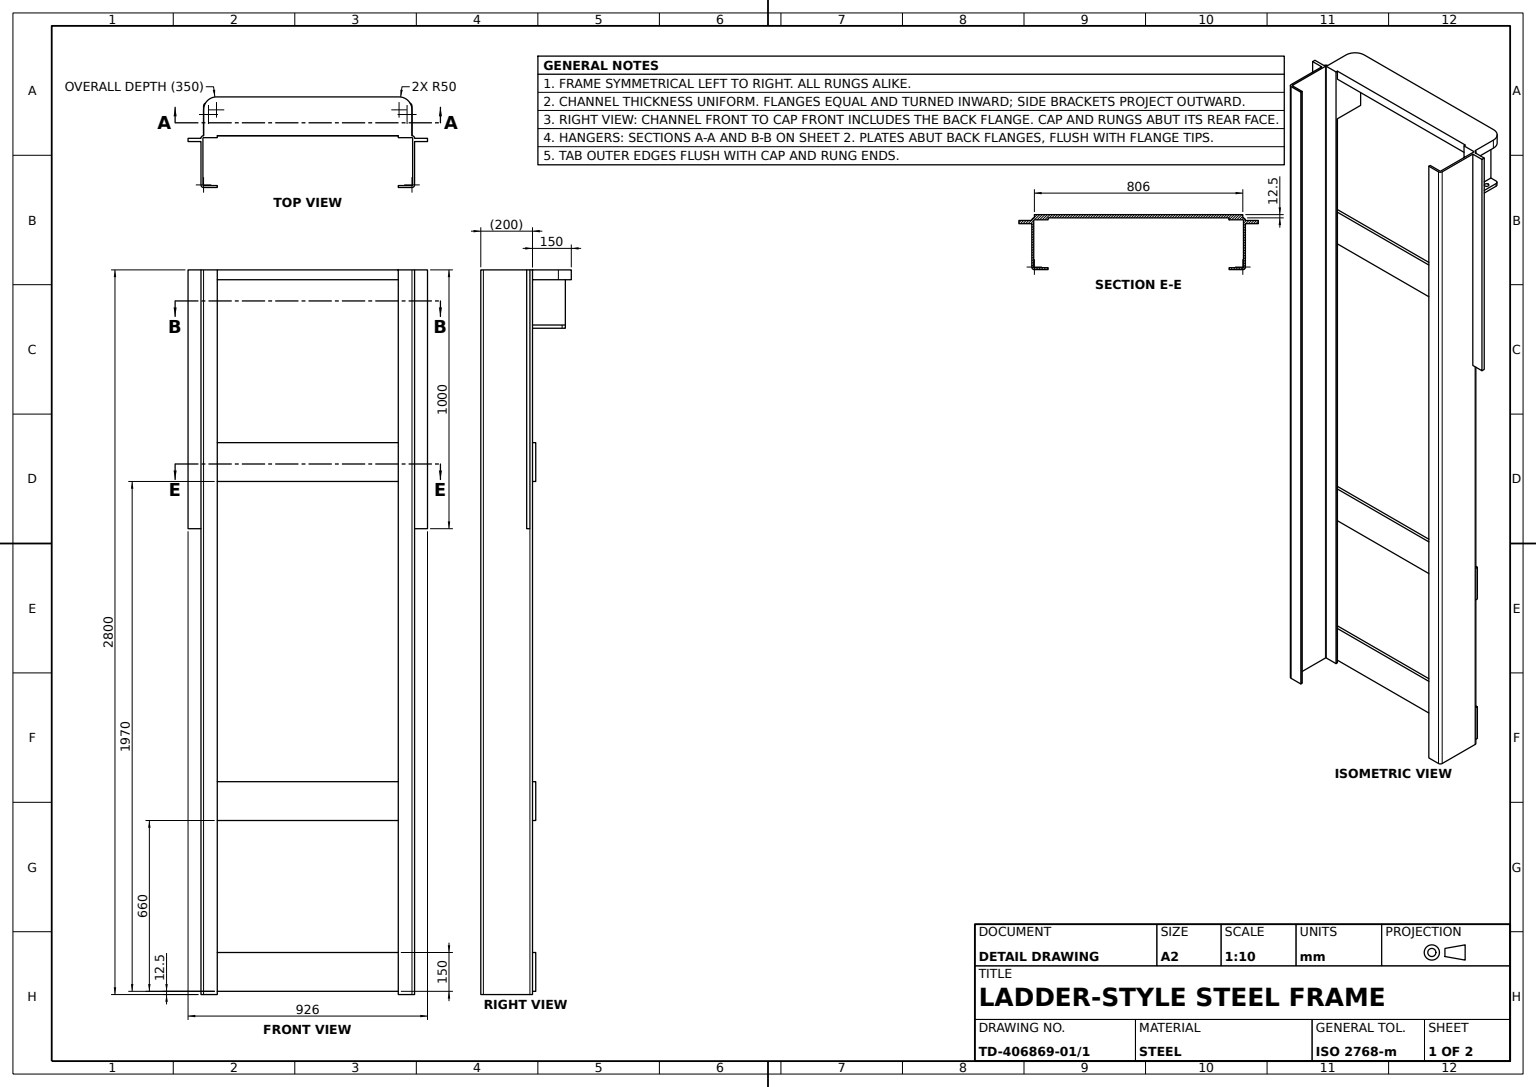
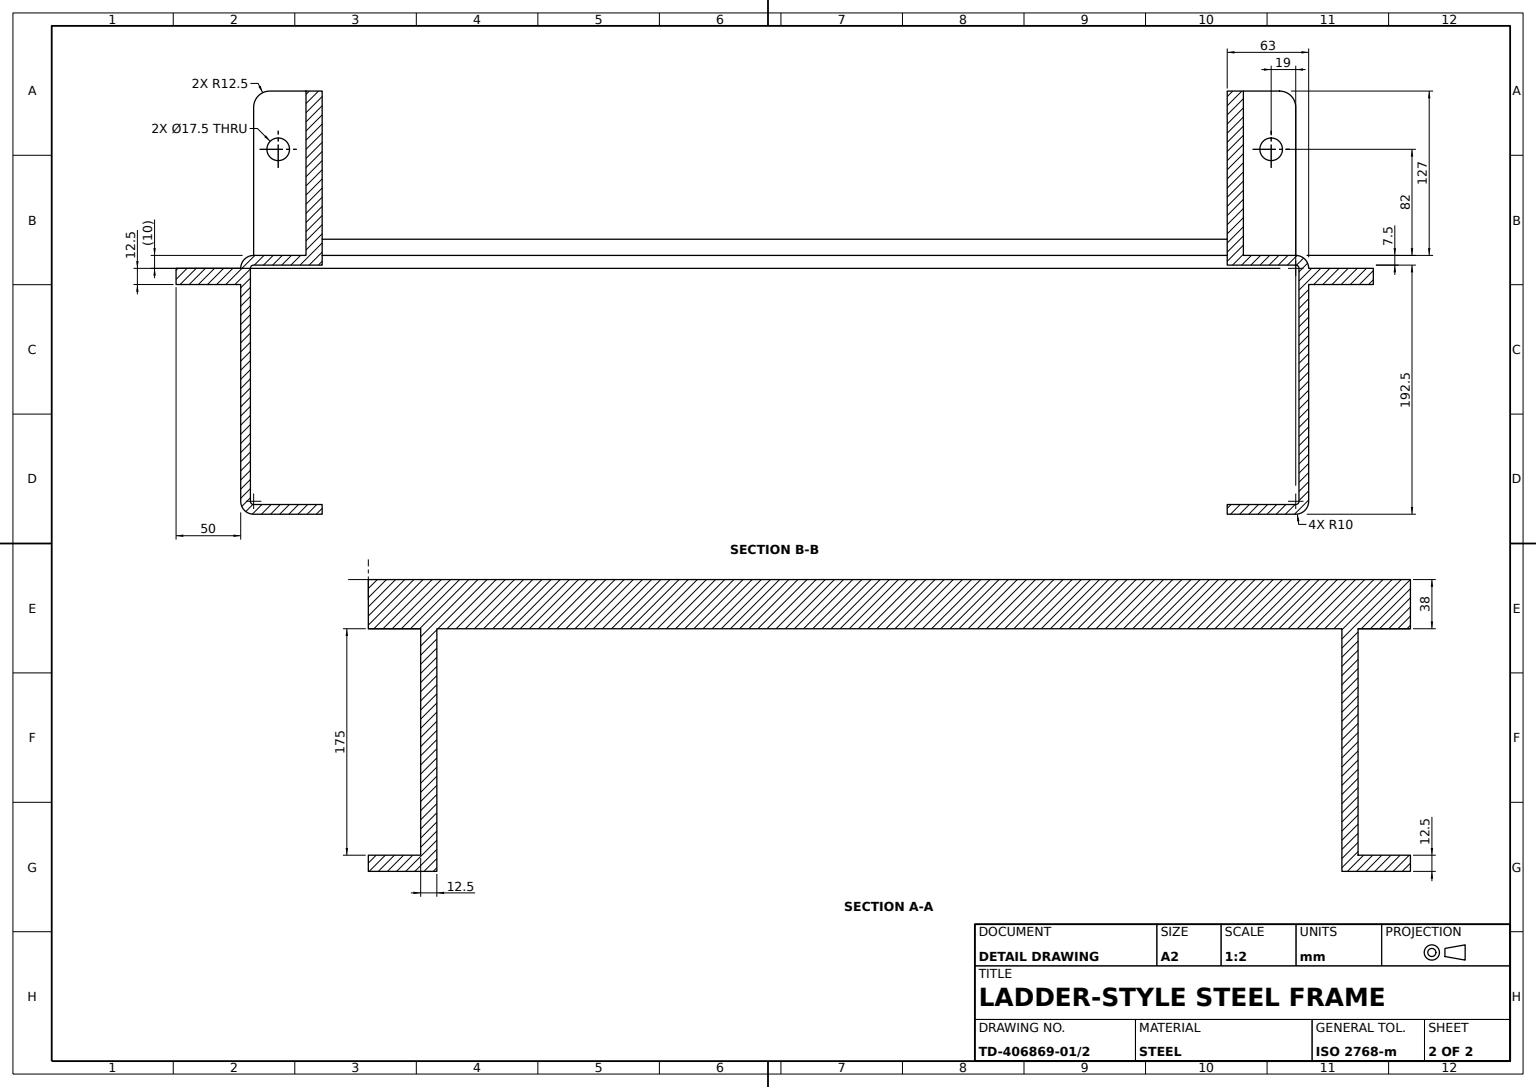
SolidWorks part; units mm, degrees
material "Plain Carbon Steel"
ref_plane "Front Plane" through (0, 0, 0) normal (0, 0, 1) x (1, 0, 0)
ref_plane "Top Plane" through (0, 0, 0) normal (0, 1, 0) x (1, 0, 0)
ref_plane "Right Plane" through (0, 0, 0) normal (1, 0, 0) x (0, 0, -1)
sketch "Side Channel Profile Sketch" plane through (0, 0, 0) normal (0, 1, 0) x (1, 0, 0)
  line L0 (0, 0) -> (413, 0) construction
  line L1 (350, 100) -> (403, 100)
  line L2 (413, 90) -> (413, -90)
  line L3 (403, -100) -> (350, -100)
  arc A0 (413, -90) -> (403, -100) centre (403, -90) cw
  arc A1 (403, 100) -> (413, 90) centre (403, 90) cw
  point P5 (413, 0)
  point P10 (413, -100)
  point P13 (413, 100)
  dimension "D4" = 10
  dimension "D1" = 413
  dimension "D2" = 200
  dimension "D3" = 63
extrude "Side Channel Rail L2800" add sketch "Side Channel Profile Sketch" along normal mid plane 2800 thin
sketch "Top Cap Sketch" plane through (0, 1400, 0) normal (0, 1, 0) x (1, 0, 0)
  line L0 (413, 90) -> (463, 90)
  line L1 (463, 90) -> (463, 77.5)
  line L2 (463, 77.5) -> (413, 77.5)
  line L3 (413, 90) -> (413, -90) construction
  line L4 (413, 77.5) -> (413, 90)
  dimension "D1" = 50
  dimension "D2" = 12.5
extrude "Top Cap Plate" add sketch "Top Cap Sketch" against normal blind 1000
mirror "Side Rail Mirror" about plane through (0, 0, 0) normal (1, 0, 0) of bodies 102
sketch "Bracket Sketch" plane through (0, 1400, 0) normal (0, 1, 0) x (1, 0, 0)
  line L0 (350, 100) -> (403, 100) construction
  line L1 (-403, 100) -> (403, 100)
  line L2 (-403, 100) -> (-403, 200)
  line L3 (-353, 250) -> (353, 250)
  line L4 (403, 100) -> (403, 200)
  arc A0 (-403, 200) -> (-353, 250) centre (-353, 200) cw
  arc A1 (353, 250) -> (403, 200) centre (353, 200) cw
  point P14 (-403, 250)
  dimension "D2" = 50
  dimension "D1" = 150
extrude "Side Bracket" add sketch "Bracket Sketch" against normal blind 38
sketch "Cross Bar Sketch" plane through (0, 0, -100) normal (0, 0, -1) x (-1, 0, 0)
  line L0 (-403, 1362) -> (-403, -1400) construction
  line L1 (-403, -1387.5) -> (403, -1387.5)
  line L2 (-403, -1387.5) -> (-403, -1237.5)
  line L3 (-403, -1237.5) -> (403, -1237.5)
  line L4 (403, -1387.5) -> (403, -1237.5)
  line L5 (403, 1362) -> (403, -1400) construction
  line L6 (-350, -1400) -> (-403, -1400) construction
  dimension "D1" = 12.5
  dimension "D2" = 150
extrude "Cross Bar" add sketch "Cross Bar Sketch" along normal blind 12.5
pattern_linear "Cross Bar Pattern 660" count 2 spacing 660 along (0, 1, 0) of "Cross Bar"
pattern_linear "Cross Bar Pattern 1970" count 2 spacing 1970 along (0, 1, 0) of "Cross Bar"
sketch "Hanger Plate Sketch" plane through (0, 1362, 0) normal (0, -1, 0) x (1, 0, 0)
  line L1 (-350, -100) -> (-362.5, -100)
  line L2 (-350, -100) -> (-350, -227)
  line L3 (-350, -227) -> (-362.5, -227)
  line L4 (-362.5, -100) -> (-362.5, -227)
  dimension "D1" = 12.5
  dimension "D2" = 127
extrude "Hanger Plate" add sketch "Hanger Plate Sketch" along normal blind 175
sketch "Hanger Tab Sketch" plane through (0, 1187, 0) normal (0, -1, 0) x (1, 0, 0)
  line L1 (-350, -100) -> (-403, -100)
  line L2 (-350, -100) -> (-350, -227)
  line L3 (-350, -227) -> (-403, -227)
  line L4 (-403, -100) -> (-403, -227)
  circle A0 centre (-384, -182) radius 8.75
  dimension "D1" = 17.5
  dimension "D2" = 19
  dimension "D3" = 82
extrude "Hanger Tab" add sketch "Hanger Tab Sketch" along normal blind 12.5
fillet "Hanger Tab Fillet R12.5" radius 12.5 1 edges at (-403, 1180.75, -227)
mirror "Side Bracket Mirror" about plane through (0, 0, 0) normal (1, 0, 0) of bodies 112
